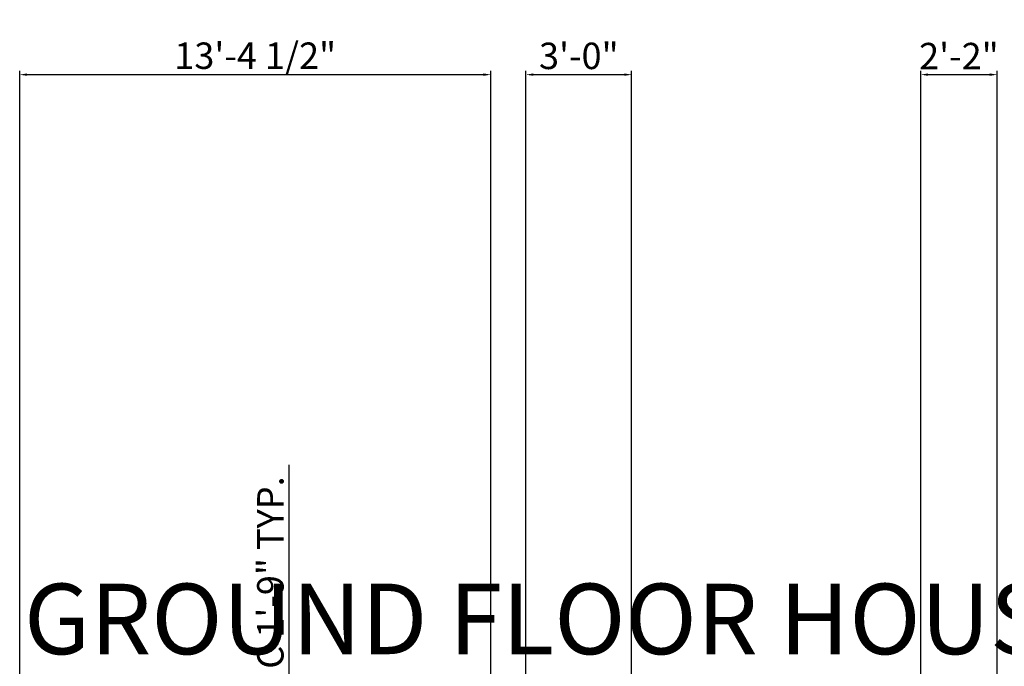
# Model space of a CAD drawing. Units: inches. Extents: x 744 to 1448, y 5126 to 6077.
# Tile 9 of 10: x 817 to 1152, y 5857 to 6077. Entities that reach past the tile are written whole.
import ezdxf

# ---------------------------------------------------------------- set-up
doc = ezdxf.new("R2010")
doc.units = ezdxf.units.IN
doc.layers.add('A-ANNO-DIMS', color=2, linetype='Continuous', lineweight=18)
doc.layers.add('A-ANNO-TEXT', color=7, linetype='Continuous', lineweight=18)
doc.styles.get("Standard").update_dxf_attribs({"font": 'arial.ttf'})
doc.dimstyles.new('ISO-25', dxfattribs={"dimtxt": 9, "dimasz": 2.5, "dimexe": 1.25, "dimexo": 0.625, "dimtad": 1, "dimlunit": 3, "dimtxsty": 'Standard', "dimcen": 2.5, "dimadec": 0, "dimazin": 0, "dimtfac": 1, "dimtmove": 0, "dimatfit": 3, "dimfxl": 1, "dimarcsym": 0})

# ---------------------------------------------------------------- blocks, each defined once
blk = doc.blocks.new('*D41')
at = {"layer": 'A-ANNO-DIMS', "color": 0, "lineweight": -2, "transparency": 16777216}
for p, q in [((908.53, 5795.32), (908.53, 5925.53)), ((911.06, 5795.32), (907.28, 5795.32)), ((908.53, 5776.82), (908.53, 5792.82)), ((911.06, 5774.32), (907.28, 5774.32))]:
    blk.add_line(p, q, dxfattribs=at)
at = {"layer": 'A-ANNO-DIMS', "color": 0, "transparency": 16777216}
for points in [[(908.12, 5792.82), (908.95, 5792.82), (908.53, 5795.32)], [(908.12, 5776.82), (908.95, 5776.82), (908.53, 5774.32)]]:
    blk.add_solid(points, dxfattribs=at)
at = {"layer": 'Defpoints', "color": 0, "transparency": 16777216}
for p in [(908.53, 5795.32), (911.68, 5795.32), (911.68, 5774.32)]:
    blk.add_point(p, dxfattribs=at)
at = {"layer": 'A-ANNO-DIMS', "color": 0, "transparency": 16777216, "insert": (903.25, 5861.67), "char_height": 9, "attachment_point": 5, "rotation": 90}
blk.add_mtext('WINDOW C 1\'-9" TYP.', dxfattribs=at)
blk = doc.blocks.new('*D55')
at = {"layer": 'A-ANNO-DIMS', "color": 0, "lineweight": -2, "transparency": 16777216}
for p, q in [((989.18, 5323.94), (989.18, 6059.61)), ((991.68, 6058.36), (1022.68, 6058.36)), ((1025.18, 5323.94), (1025.18, 6059.61))]:
    blk.add_line(p, q, dxfattribs=at)
at = {"layer": 'A-ANNO-DIMS', "color": 0, "transparency": 16777216}
for points in [[(991.68, 6058.78), (991.68, 6057.95), (989.18, 6058.36)], [(1022.68, 6058.78), (1022.68, 6057.95), (1025.18, 6058.36)]]:
    blk.add_solid(points, dxfattribs=at)
at = {"layer": 'Defpoints', "color": 0, "transparency": 16777216}
for p in [(1025.18, 6058.36), (989.18, 5323.32), (1025.18, 5323.32)]:
    blk.add_point(p, dxfattribs=at)
at = {"layer": 'A-ANNO-DIMS', "color": 0, "transparency": 16777216, "insert": (1007.18, 6063.59), "char_height": 9, "attachment_point": 5}
blk.add_mtext('3\'-0"', dxfattribs=at)
blk = doc.blocks.new('*D57')
at = {"layer": 'A-ANNO-DIMS', "color": 0, "lineweight": -2, "transparency": 16777216}
for p, q in [((1123.68, 5672.44), (1123.68, 6059.61)), ((1126.18, 6058.36), (1147.18, 6058.36)), ((1149.68, 5672.44), (1149.68, 6059.61))]:
    blk.add_line(p, q, dxfattribs=at)
at = {"layer": 'A-ANNO-DIMS', "color": 0, "transparency": 16777216}
for points in [[(1126.18, 6058.78), (1126.18, 6057.95), (1123.68, 6058.36)], [(1147.18, 6058.78), (1147.18, 6057.95), (1149.68, 6058.36)]]:
    blk.add_solid(points, dxfattribs=at)
at = {"layer": 'Defpoints', "color": 0, "transparency": 16777216}
for p in [(1149.68, 6058.36), (1123.68, 5671.82), (1149.68, 5671.82)]:
    blk.add_point(p, dxfattribs=at)
at = {"layer": 'A-ANNO-DIMS', "color": 0, "transparency": 16777216, "insert": (1136.68, 6063.51), "char_height": 9, "attachment_point": 5}
blk.add_mtext('2\'-2"', dxfattribs=at)
blk = doc.blocks.new('*D62')
at = {"layer": 'A-ANNO-DIMS', "color": 0, "lineweight": -2, "transparency": 16777216}
for p, q in [((816.68, 5262.94), (816.68, 6059.61)), ((819.18, 6058.36), (974.68, 6058.36)), ((977.18, 5262.94), (977.18, 6059.61))]:
    blk.add_line(p, q, dxfattribs=at)
at = {"layer": 'A-ANNO-DIMS', "color": 0, "transparency": 16777216}
for points in [[(819.18, 6058.78), (819.18, 6057.95), (816.68, 6058.36)], [(974.68, 6058.78), (974.68, 6057.95), (977.18, 6058.36)]]:
    blk.add_solid(points, dxfattribs=at)
at = {"layer": 'Defpoints', "color": 0, "transparency": 16777216}
for p in [(977.18, 6058.36), (816.68, 5262.32), (977.18, 5262.32)]:
    blk.add_point(p, dxfattribs=at)
at = {"layer": 'A-ANNO-DIMS', "color": 0, "transparency": 16777216, "insert": (896.93, 6063.64), "char_height": 9, "attachment_point": 5}
blk.add_mtext('13\'-4 1/2"', dxfattribs=at)

msp = doc.modelspace()

# ---------------------------------------------------------------- texts
at = {"layer": 'A-ANNO-TEXT', "insert": (818.158, 5885.054), "char_height": 24, "attachment_point": 1}
msp.add_mtext_dynamic_manual_height_columns('GROUND FLOOR HOUSE PLAN', width=502.97243, gutter_width=12.5, heights=[0], dxfattribs=at)

# ---------------------------------------------------------------- dimensions: what is measured, and where the dimension line sits
at = {"layer": 'A-ANNO-DIMS'}
for base, p1, p2, picture, middle in [((977.184, 6058.363), (816.684, 5262.316), (977.184, 5262.316), '*D62', (896.934, 6063.645)), ((1025.184, 6058.363), (989.184, 5323.316), (1025.184, 5323.316), '*D55', (1007.184, 6063.586)), ((1149.684, 6058.363), (1123.684, 5671.816), (1149.684, 5671.816), '*D57', (1136.684, 6063.507))]:
    dim = msp.add_linear_dim(base=base, p1=p1, p2=p2, dimstyle='ISO-25', override={"dimdec": 1, "dimlfac": 1, "dimrnd": 0, "dimzin": 1, "dimdsep": 46, "dimlunit": 4, "dimfrac": 2}, dxfattribs=at)
    dim.commit()
    dim.dimension.update_dxf_attribs({"geometry": picture, "text_midpoint": middle})
dim = msp.add_linear_dim(base=(908.534, 5795.316), p1=(911.684, 5774.316), p2=(911.684, 5795.316), angle=90, text='WINDOW C <> TYP.', dimstyle='ISO-25', override={"dimdec": 1, "dimlfac": 1, "dimrnd": 0, "dimzin": 1, "dimdsep": 46, "dimlunit": 4, "dimfrac": 2}, dxfattribs=at)
dim.commit()
dim.dimension.update_dxf_attribs({"geometry": '*D41', "text_midpoint": (903.253, 5861.671)})

doc.saveas('drawing.dxf')
